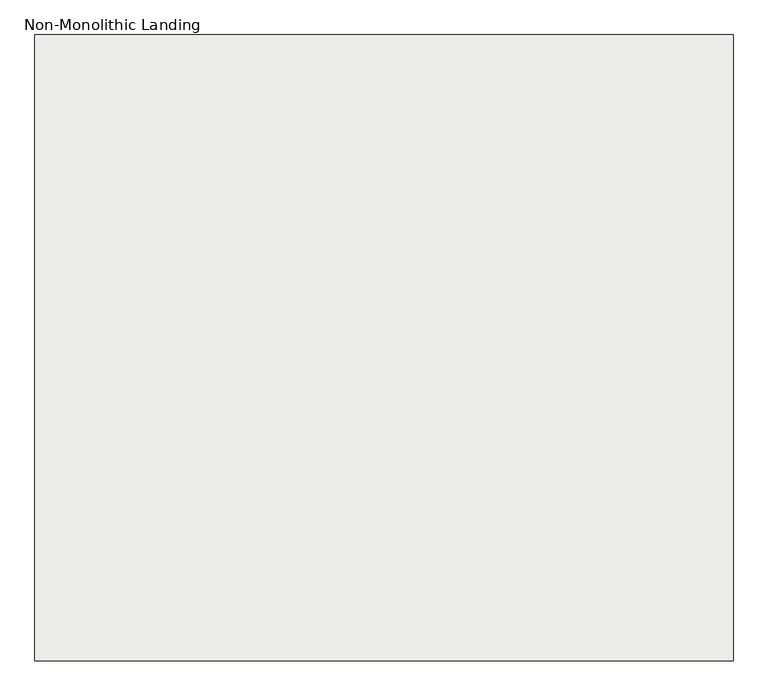
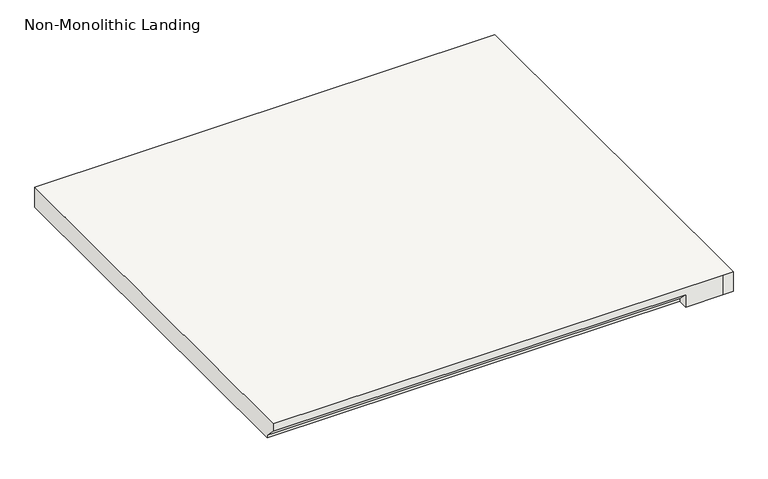
"""IFC4 building model written with IfcOpenShell, lengths in millimetres: slab geometry, Non-Monolithic Landing."""

from ifc_helpers import new_model, si_unit, origin, place, context, project, spatial, faceted_brep, source, transform, mapped, element, save


def non_monolithic_landing_c2e7054d(model_context):
    return source(origin(), model_context, "Body", "Brep", [
        faceted_brep([(-7815.6002526, 11195.5128362, 4705.35), (-7815.6002526, 11220.9128362, 4679.95), (-6818.6502526, 11220.9128362, 4679.95), (-6818.6502526, 11195.5128362, 4705.35), (-6729.7502524, 11195.5128362, 4724.4), (-6704.3502524, 11195.5128362, 4724.4), (-6704.3502524, 12192.4628362, 4724.4), (-6729.7502524, 12192.4628362, 4724.4), (-7815.6002526, 12192.4628362, 4724.4), (-7815.6002526, 11195.5128362, 4724.4), (-6818.6502526, 11220.9128362, 4673.6), (-7815.6002526, 11220.9128362, 4673.6), (-7815.6002526, 12192.4628362, 4673.6), (-6729.7502524, 12192.4628362, 4673.6), (-6704.3502524, 12192.4628362, 4673.6), (-6704.3502524, 11195.5128362, 4673.6), (-6729.7502524, 11195.5128362, 4673.6), (-6818.6502526, 11195.5128362, 4673.6)], [[[0, 1, 2, 3]], [[4, 5, 6, 7, 8, 9]], [[10, 11, 12, 13, 14, 15, 16, 17]], [[11, 10, 2, 1]], [[10, 17, 3, 2]], [[4, 9, 0, 3, 17, 16]], [[5, 4, 16, 15]], [[6, 5, 15, 14]], [[7, 6, 14, 13]], [[8, 7, 13, 12]], [[9, 8, 12, 11, 1, 0]]]),
    ])


if __name__ == "__main__":
    model = new_model("IFC4")
    model_context = context("Model", 3, world=origin())
    ifc_project = project(units=[si_unit("LENGTHUNIT", "METRE", prefix="MILLI")], contexts=[model_context])
    site = spatial("IfcSite", under=ifc_project)
    building = spatial("IfcBuilding", under=site)
    placement = place(None, origin())
    non_monolithic_landing_shape = non_monolithic_landing_c2e7054d(model_context)
    element("IfcSlab", 1, ObjectType="Non-Monolithic Landing", at=placement, inside=building, context=model_context, shape_type="MappedRepresentation", body=[
        mapped(non_monolithic_landing_shape, transform((0.0, 0.0, 0.0), x_axis=(1.0, 0.0, 0.0), y_axis=(0.0, 1.0, 0.0), z_axis=(0.0, 0.0, 1.0))),
    ])
    save(model, "model.ifc")
